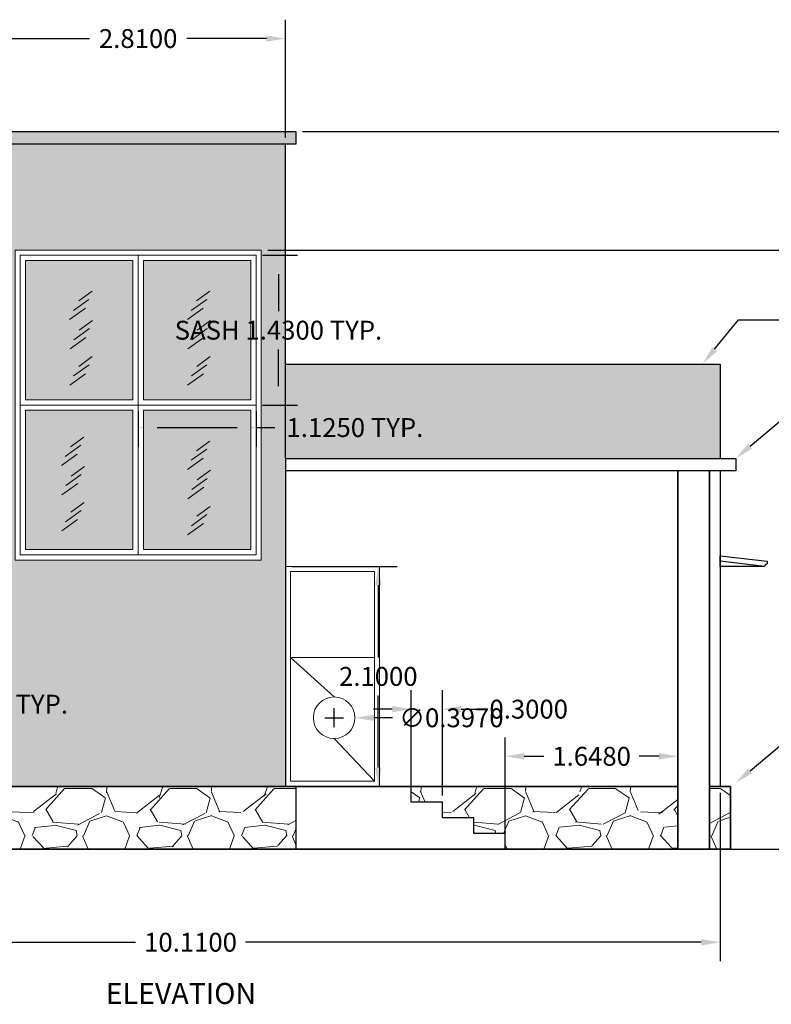
# Model space of a CAD drawing. Units: metres. Extents: x 5.2 to 41.7, y 12.2 to 37.4.
# Tile 2 of 6: x 12.3 to 19.4, y 28 to 37.4. Entities that reach past the tile are written whole.
import ezdxf
from ezdxf import colors
from ezdxf.entities.mleader import LeaderData, LeaderLine
from ezdxf.math import Vec2, Vec3

# ---------------------------------------------------------------- set-up
doc = ezdxf.new("R2010")
doc.units = ezdxf.units.M
doc.header["$MEASUREMENT"] = 0
for name, color, linetype, lineweight in [('A-ANNO-DIMS', 2, 'Continuous', 18), ('A-ANNO-TEXT', 3, 'Continuous', 18), ('A-COLS', 1, 'Continuous', 35), ('A-DOOR', 4, 'Continuous', 18), ('A-ELEV', 7, 'Continuous', 25), ('A-ELEV-PATT', 9, 'Continuous', 13), ('A-FLOR-PLIN', 7, 'Continuous', 25), ('A-FLOR-STRS', 7, 'Continuous', 25), ('A-GLAZ-PATT', 151, 'Continuous', 13), ('A-ROOF', 7, 'Continuous', 25), ('C-TOPO', 7, 'Continuous', 25)]:
    doc.layers.add(name, color=color, linetype=linetype, lineweight=lineweight)
doc.layers.add('A-GLAZ', color=51, linetype='Continuous', lineweight=18, true_color=0xf7f281)
doc.layers.add('A-PLIN-PATT', color=251, linetype='Continuous', lineweight=13, true_color=0x636466)
doc.styles.get("Standard").update_dxf_attribs({"font": 'arial.ttf'})
doc.dimstyles.get("Standard").update_dxf_attribs({"dimtxt": 0.18, "dimasz": 0.18, "dimexe": 0.18, "dimexo": 0.0625, "dimgap": 0.09, "dimtad": 0, "dimtih": 1, "dimtoh": 1, "dimdec": 4, "dimzin": 0, "dimdsep": 46, "dimtxsty": 'Standard', "dimcen": 0.09, "dimadec": 0, "dimazin": 0, "dimtfac": 1, "dimtdec": 4, "dimtofl": 0, "dimtmove": 0, "dimatfit": 3, "dimfxl": 1, "dimtolj": 1, "dimtzin": 0, "dimarcsym": 0})

# ---------------------------------------------------------------- blocks, each defined once
blk = doc.blocks.new('GLASS-REFLECTION')
for p, q in [((0.0369433649416564, 0.0871027572389061), (0.184953556568928, 0.1937230376420551)), ((0.08809580488861, 0.178305383476971), (0.2148507561325843, 0.2711338394228626)), ((0.000485723746344, -2.27863267348e-05), (0.1515279092010928, 0.1087816141597138))]:
    blk.add_line(p, q)
blk = doc.blocks.new('SASH-ELEV-TOWER')
for points in [[(-0.0004402787265363, 1.429717152800996), (1.12455972127346, 1.429717152800996), (1.12455972127346, -0.0002828471990028), (-0.0004402787265363, -0.0002828471990028)], [(0.0495597212734644, 1.379717152800999), (1.074559721273459, 1.379717152800999), (1.074559721273459, 0.0497171528009943), (0.0495597212734644, 0.0497171528009943)]]:
    blk.add_lwpolyline(points, close=True)
blk = doc.blocks.new('*D20')
at = {"layer": 'A-ANNO-DIMS', "color": 0, "lineweight": -2, "transparency": 16777216}
for p, q in [((14.58205972127346, 35.11471715280102), (14.91405972127346, 35.11471715280102)), ((14.73405972127346, 34.93471715280102), (14.73405972127346, 34.58284812142313)), ((14.73405972127346, 33.86471715280102), (14.73405972127346, 34.21658618417892)), ((14.58205972127346, 33.68471715280102), (14.91405972127346, 33.68471715280102))]:
    blk.add_line(p, q, dxfattribs=at)
at = {"layer": 'A-ANNO-DIMS', "color": 0, "lineweight": 25, "transparency": 16777216}
for points in [[(14.70405972127346, 34.93471715280102), (14.76405972127346, 34.93471715280102), (14.73405972127346, 35.11471715280102)], [(14.70405972127346, 33.86471715280102), (14.76405972127346, 33.86471715280102), (14.73405972127346, 33.68471715280102)]]:
    blk.add_solid(points, dxfattribs=at)
at = {"layer": 'Defpoints', "color": 0, "lineweight": 25, "transparency": 16777216}
for p in [(14.51955972127346, 35.11471715280102), (14.73405972127346, 35.11471715280102), (14.51955972127346, 33.68471715280102)]:
    blk.add_point(p, dxfattribs=at)
at = {"layer": 'A-ANNO-DIMS', "color": 0, "transparency": 16777216, "insert": (14.73405972127347, 34.39971715280102), "char_height": 0.18, "attachment_point": 5}
blk.add_mtext('\\A1;SASH 1.4300 TYP.', dxfattribs=at)
blk = doc.blocks.new('*D21')
at = {"layer": 'A-ANNO-DIMS', "color": 0, "lineweight": -2, "transparency": 16777216}
for p, q in [((13.39455972127345, 33.62221715280101), (13.39455972127345, 33.29021715280101)), ((14.51955972127345, 33.62221715280101), (14.51955972127345, 33.29021715280101)), ((13.57455972127345, 33.47021715280101), (14.33955972127345, 33.47021715280101)), ((14.51955972127345, 33.47021715280101), (14.69955972127345, 33.47021715280101))]:
    blk.add_line(p, q, dxfattribs=at)
at = {"layer": 'A-ANNO-DIMS', "color": 0, "lineweight": 25, "transparency": 16777216}
for points in [[(13.57455972127345, 33.50021715280101), (13.57455972127345, 33.44021715280101), (13.39455972127345, 33.47021715280101)], [(14.33955972127345, 33.50021715280101), (14.33955972127345, 33.44021715280101), (14.51955972127345, 33.47021715280101)]]:
    blk.add_solid(points, dxfattribs=at)
at = {"layer": 'Defpoints', "color": 0, "lineweight": 25, "transparency": 16777216}
for p in [(13.39455972127345, 33.68471715280101), (14.51955972127345, 33.68471715280101), (14.51955972127345, 33.47021715280101)]:
    blk.add_point(p, dxfattribs=at)
at = {"layer": 'A-ANNO-DIMS', "color": 0, "transparency": 16777216, "insert": (15.46388441431574, 33.47021715280101), "char_height": 0.18, "attachment_point": 5}
blk.add_mtext('\\A1;1.1250 TYP.', dxfattribs=at)
blk = doc.blocks.new('*D23')
at = {"layer": 'A-ANNO-DIMS', "color": 0, "lineweight": -2, "transparency": 16777216}
for p, q in [((10.56955972127346, 30.93221715280099), (10.56955972127346, 30.64971715280099)), ((11.11955972127346, 30.93221715280099), (11.11955972127346, 30.64971715280099)), ((10.74955972127346, 30.82971715280099), (10.93955972127346, 30.82971715280099)), ((11.11955972127346, 30.82971715280099), (11.29955972127346, 30.82971715280099))]:
    blk.add_line(p, q, dxfattribs=at)
at = {"layer": 'A-ANNO-DIMS', "color": 0, "lineweight": 25, "transparency": 16777216}
for points in [[(10.74955972127346, 30.85971715280099), (10.74955972127346, 30.79971715280099), (10.56955972127346, 30.82971715280099)], [(10.93955972127346, 30.85971715280099), (10.93955972127346, 30.79971715280099), (11.11955972127346, 30.82971715280099)]]:
    blk.add_solid(points, dxfattribs=at)
at = {"layer": 'Defpoints', "color": 0, "lineweight": 25, "transparency": 16777216}
for p in [(10.56955972127346, 30.99471715280099), (11.11955972127346, 30.99471715280099), (11.11955972127346, 30.82971715280099)]:
    blk.add_point(p, dxfattribs=at)
at = {"layer": 'A-ANNO-DIMS', "color": 0, "transparency": 16777216, "insert": (12.07235644705791, 30.82971715280099), "char_height": 0.18, "attachment_point": 5}
blk.add_mtext('\\A1;0.5500 TYP.', dxfattribs=at)
blk = doc.blocks.new('*D37')
at = {"layer": 'A-ANNO-DIMS', "color": 0, "lineweight": -2, "transparency": 16777216}
for p, q in [((8.83956, 29.982217), (8.83956, 28.377217)), ((18.94956, 29.982217), (18.94956, 28.377217)), ((9.01956, 28.557217), (13.36978510231924, 28.557217)), ((18.76956, 28.557217), (14.41933489768076, 28.557217))]:
    blk.add_line(p, q, dxfattribs=at)
at = {"layer": 'A-ANNO-DIMS', "color": 0, "lineweight": 25, "transparency": 16777216}
for points in [[(9.01956, 28.587217), (9.01956, 28.527217), (8.83956, 28.557217)], [(18.76956, 28.587217), (18.76956, 28.527217), (18.94956, 28.557217)]]:
    blk.add_solid(points, dxfattribs=at)
at = {"layer": 'Defpoints', "color": 0, "lineweight": 25, "transparency": 16777216}
for p in [(8.83956, 30.044717), (18.94956, 30.044717), (18.94956, 28.557217)]:
    blk.add_point(p, dxfattribs=at)
at = {"layer": 'A-ANNO-DIMS', "color": 0, "transparency": 16777216, "insert": (13.89456, 28.557217), "char_height": 0.18, "attachment_point": 5}
blk.add_mtext('\\A1;10.1100', dxfattribs=at)
blk = doc.blocks.new('*D38')
at = {"layer": 'A-ANNO-DIMS', "color": 0, "lineweight": -2, "transparency": 16777216}
for p, q in [((14.96206, 36.29607500000002), (22.42460000000001, 36.29607500000002)), ((22.24460000000001, 36.11607500000002), (22.24460000000001, 33.05229913778993)), ((22.24460000000001, 29.62471700000002), (22.24460000000001, 32.68849286221012)), ((21.4196, 29.44471700000002), (22.42460000000001, 29.44471700000002))]:
    blk.add_line(p, q, dxfattribs=at)
at = {"layer": 'A-ANNO-DIMS', "color": 0, "lineweight": 25, "transparency": 16777216}
for points in [[(22.21460000000001, 36.11607500000002), (22.27460000000001, 36.11607500000002), (22.24460000000001, 36.29607500000002)], [(22.21460000000001, 29.62471700000002), (22.27460000000001, 29.62471700000002), (22.24460000000001, 29.44471700000002)]]:
    blk.add_solid(points, dxfattribs=at)
at = {"layer": 'Defpoints', "color": 0, "lineweight": 25, "transparency": 16777216}
for p in [(14.89956, 36.29607500000002), (22.24460000000001, 36.29607500000002), (21.35710000000001, 29.44471700000002)]:
    blk.add_point(p, dxfattribs=at)
at = {"layer": 'A-ANNO-DIMS', "color": 0, "transparency": 16777216, "insert": (22.24460000000002, 32.87039600000001), "char_height": 0.18, "attachment_point": 5}
blk.add_mtext('\\A1;6.8514', dxfattribs=at)
blk = doc.blocks.new('*D41')
at = {"layer": 'A-ANNO-DIMS', "color": 0, "lineweight": -2, "transparency": 16777216}
for p, q in [((11.98956, 36.238575), (11.98956, 37.363575)), ((14.79956, 36.238575), (14.79956, 37.363575)), ((12.16956, 37.183575), (12.92970324693042, 37.183575)), ((14.61956, 37.183575), (13.85941675306957, 37.183575))]:
    blk.add_line(p, q, dxfattribs=at)
at = {"layer": 'A-ANNO-DIMS', "color": 0, "lineweight": 25, "transparency": 16777216}
for points in [[(12.16956, 37.213575), (12.16956, 37.153575), (11.98956, 37.183575)], [(14.61956, 37.213575), (14.61956, 37.153575), (14.79956, 37.183575)]]:
    blk.add_solid(points, dxfattribs=at)
at = {"layer": 'Defpoints', "color": 0, "lineweight": 25, "transparency": 16777216}
for p in [(14.79956, 37.183575), (11.98956, 36.176075), (14.79956, 36.176075)]:
    blk.add_point(p, dxfattribs=at)
at = {"layer": 'A-ANNO-DIMS', "color": 0, "transparency": 16777216, "insert": (13.39456, 37.183575), "char_height": 0.18, "attachment_point": 5}
blk.add_mtext('\\A1;2.8100', dxfattribs=at)
blk = doc.blocks.new('*D44')
at = {"layer": 'A-ANNO-DIMS', "color": 0, "lineweight": -2, "transparency": 16777216}
for p, q in [((14.86206000000001, 32.14471700000002), (15.86706000000001, 32.14471700000002)), ((15.68706000000001, 31.96471700000002), (15.68706000000001, 31.27662013778992)), ((15.68706000000001, 30.22471700000001), (15.68706000000001, 30.91281386221011)), ((14.86206000000001, 30.04471700000002), (15.86706000000001, 30.04471700000002))]:
    blk.add_line(p, q, dxfattribs=at)
at = {"layer": 'A-ANNO-DIMS', "color": 0, "lineweight": 25, "transparency": 16777216}
for points in [[(15.65706000000001, 31.96471700000002), (15.71706000000001, 31.96471700000002), (15.68706000000001, 32.14471700000002)], [(15.65706000000001, 30.22471700000001), (15.71706000000001, 30.22471700000001), (15.68706000000001, 30.04471700000002)]]:
    blk.add_solid(points, dxfattribs=at)
at = {"layer": 'Defpoints', "color": 0, "lineweight": 25, "transparency": 16777216}
for p in [(14.79956, 32.14471700000002), (14.79956, 30.04471700000002), (15.68706000000001, 30.04471700000002)]:
    blk.add_point(p, dxfattribs=at)
at = {"layer": 'A-ANNO-DIMS', "color": 0, "transparency": 16777216, "insert": (15.68706000000002, 31.094717), "char_height": 0.18, "attachment_point": 5}
blk.add_mtext('\\A1;2.1000', dxfattribs=at)
blk = doc.blocks.new('*D45')
at = {"layer": 'A-ANNO-DIMS', "color": 0, "lineweight": -2, "transparency": 16777216}
for p, q in [((14.96206, 36.29607500000002), (22.42460000000001, 36.29607500000002)), ((22.24460000000001, 36.11607500000002), (22.24460000000001, 35.91236052933155)), ((22.24460000000001, 35.34471700000003), (22.24460000000001, 35.54843147066851)), ((14.63206, 35.16471700000002), (22.42460000000001, 35.16471700000002))]:
    blk.add_line(p, q, dxfattribs=at)
at = {"layer": 'A-ANNO-DIMS', "color": 0, "lineweight": 25, "transparency": 16777216}
for points in [[(22.21460000000001, 36.11607500000002), (22.27460000000001, 36.11607500000002), (22.24460000000001, 36.29607500000002)], [(22.21460000000001, 35.34471700000003), (22.27460000000001, 35.34471700000003), (22.24460000000001, 35.16471700000002)]]:
    blk.add_solid(points, dxfattribs=at)
at = {"layer": 'Defpoints', "color": 0, "lineweight": 25, "transparency": 16777216}
for p in [(14.89956, 36.29607500000002), (22.24460000000001, 36.29607500000002), (14.56956, 35.16471700000002)]:
    blk.add_point(p, dxfattribs=at)
at = {"layer": 'A-ANNO-DIMS', "color": 0, "transparency": 16777216, "insert": (22.24460000000002, 35.73039600000001), "char_height": 0.18, "attachment_point": 5}
blk.add_mtext('\\A1;1.1314', dxfattribs=at)
blk = doc.blocks.new('*D76')
at = {"layer": 'A-ANNO-DIMS', "color": 0, "lineweight": -2, "transparency": 16777216}
for p, q in [((15.99956, 29.957217), (15.99956, 30.962217)), ((16.29956, 29.957217), (16.29956, 30.962217)), ((15.81956, 30.782217), (15.63956, 30.782217)), ((16.47956, 30.782217), (16.65956, 30.782217))]:
    blk.add_line(p, q, dxfattribs=at)
at = {"layer": 'A-ANNO-DIMS', "color": 0, "lineweight": 25, "transparency": 16777216}
for points in [[(15.81956, 30.812217), (15.81956, 30.752217), (15.99956, 30.782217)], [(16.47956, 30.812217), (16.47956, 30.752217), (16.29956, 30.782217)]]:
    blk.add_solid(points, dxfattribs=at)
at = {"layer": 'Defpoints', "color": 0, "lineweight": 25, "transparency": 16777216}
for p in [(16.29956, 30.782217), (15.99956, 29.894717), (16.29956, 29.894717)]:
    blk.add_point(p, dxfattribs=at)
at = {"layer": 'A-ANNO-DIMS', "color": 0, "transparency": 16777216, "insert": (17.12288196452933, 30.782217), "char_height": 0.18, "attachment_point": 5}
blk.add_mtext('\\A1;0.3000', dxfattribs=at)
blk = doc.blocks.new('*D77')
at = {"layer": 'A-ANNO-DIMS', "color": 0, "lineweight": -2, "transparency": 16777216}
for p, q in [((16.89956, 29.507217), (16.89956, 30.512217)), ((18.54752, 29.507217), (18.54752, 30.512217)), ((17.07956, 30.332217), (17.26869006821282, 30.332217)), ((18.36752, 30.332217), (18.17838993178717, 30.332217))]:
    blk.add_line(p, q, dxfattribs=at)
at = {"layer": 'A-ANNO-DIMS', "color": 0, "lineweight": 25, "transparency": 16777216}
for points in [[(17.07956, 30.362217), (17.07956, 30.302217), (16.89956, 30.332217)], [(18.36752, 30.362217), (18.36752, 30.302217), (18.54752, 30.332217)]]:
    blk.add_solid(points, dxfattribs=at)
at = {"layer": 'Defpoints', "color": 0, "lineweight": 25, "transparency": 16777216}
for p in [(18.54752, 30.332217), (16.89956, 29.444717), (18.54752, 29.444717)]:
    blk.add_point(p, dxfattribs=at)
at = {"layer": 'A-ANNO-DIMS', "color": 0, "transparency": 16777216, "insert": (17.72354, 30.332217), "char_height": 0.18, "attachment_point": 5}
blk.add_mtext('\\A1;1.6480', dxfattribs=at)
blk = doc.blocks.new('*D96')
at = {"layer": 'A-ANNO-DIMS', "color": 0, "lineweight": -2, "transparency": 16777216}
for p, q in [((15.26549799999999, 30.61012199999999), (15.26549799999999, 30.79012199999999)), ((15.175498, 30.700122), (15.355498, 30.700122)), ((15.82400293200936, 30.69977874616909), (15.64400296600468, 30.69988937308454))]:
    blk.add_line(p, q, dxfattribs=at)
at = {"layer": 'A-ANNO-DIMS', "color": 0, "lineweight": 25, "transparency": 16777216}
blk.add_solid([(15.64402140382392, 30.72988936741866), (15.64398452818543, 30.66988937875043), (15.464003, 30.7)], dxfattribs=at)
at = {"layer": 'Defpoints', "color": 0, "lineweight": 25, "transparency": 16777216}
for p in [(15.066993, 30.70024399999999), (15.464003, 30.7)]:
    blk.add_point(p, dxfattribs=at)
at = {"layer": 'A-ANNO-DIMS', "color": 0, "transparency": 16777216, "insert": (16.38524440540635, 30.69977874616909), "char_height": 0.18, "attachment_point": 5}
blk.add_mtext('\\A1;∅0.3970', dxfattribs=at)

msp = doc.modelspace()

# ---------------------------------------------------------------- hatches: boundary and pattern name
at = {"layer": 'A-ELEV-PATT'}
h = msp.add_hatch(color=256, dxfattribs=at)
h.dxf.hatch_style = 1
h.paths.add_polyline_path([(14.89955972127346, 36.29607479937437), (11.88955972127345, 36.29607479937437), (11.88955972127345, 36.17607479937438), (14.89955972127346, 36.17607479937438)])
h.paths.add_polyline_path([(11.98955972127346, 34.07607479937438), (8.839559721273464, 34.07607479937438), (8.839559721273464, 33.17607479937438), (11.98955972127346, 33.17607479937438)])
h.paths.add_polyline_path([(18.94955972127346, 34.07607479937438), (14.79955972127346, 34.07607479937438), (14.79955972127346, 33.17607479937438), (18.94955972127346, 33.17607479937438)])
h = msp.add_hatch(color=256, dxfattribs=at)
h.dxf.hatch_style = 1
h.paths.add_polyline_path([(14.79955972127346, 32.144717152801), (14.79955972127346, 33.17607479937438), (14.79955972127346, 36.17607479937438), (11.98955972127346, 36.17607479937438), (11.98955972127346, 33.17607479937438), (11.98955972127346, 30.04471715280099), (14.79955972127346, 30.044717152801)])
h.paths.add_polyline_path([(12.21955972127346, 32.204717152801), (12.21955972127346, 35.164717152801), (14.56955972127346, 35.164717152801), (14.56955972127346, 32.204717152801)], flags=16)
h.paths.add_polyline_path([(12.26955972127346, 32.254717152801), (12.26955972127346, 33.684717152801), (12.26955972127346, 35.114717152801), (13.39455972127346, 35.114717152801), (14.51955972127345, 35.114717152801), (14.51955972127345, 33.684717152801), (14.51955972127345, 32.254717152801), (13.39455972127346, 32.254717152801)], flags=0)
h.paths.add_polyline_path([(12.26955972127346, 32.25471715280099), (12.26955972127346, 35.114717152801), (14.51955972127346, 35.114717152801), (14.51955972127346, 32.25471715280099)], flags=0)
h.paths.add_polyline_path([(12.31955972127346, 32.304717152801), (12.31955972127346, 33.63471715280101), (13.34455972127346, 33.63471715280101), (13.34455972127346, 32.304717152801)], flags=0)
h.paths.add_polyline_path([(13.44455972127346, 32.304717152801), (13.44455972127346, 33.63471715280101), (14.46955972127345, 33.63471715280101), (14.46955972127345, 32.304717152801)], flags=0)
h.paths.add_polyline_path([(12.31955972127346, 33.734717152801), (12.31955972127346, 35.064717152801), (13.34455972127346, 35.064717152801), (13.34455972127346, 33.734717152801)], flags=0)
h.paths.add_polyline_path([(13.44455972127346, 33.734717152801), (13.44455972127346, 35.064717152801), (14.46955972127345, 35.064717152801), (14.46955972127345, 33.734717152801)], flags=0)
h = msp.add_hatch(color=256, dxfattribs=at)
h.dxf.hatch_style = 1
h.paths.add_polyline_path([(14.79955972127346, 32.144717152801), (14.79955972127346, 33.17607479937438), (14.79955972127346, 36.17607479937438), (11.98955972127346, 36.17607479937438), (11.98955972127346, 33.17607479937438), (11.98955972127346, 30.04471715280099), (14.79955972127346, 30.044717152801)])
h.paths.add_polyline_path([(12.21955972127346, 32.204717152801), (12.21955972127346, 35.164717152801), (14.56955972127346, 35.164717152801), (14.56955972127346, 32.204717152801)], flags=16)
h.paths.add_polyline_path([(13.39455972127346, 32.254717152801), (12.26955972127346, 32.254717152801), (12.26955972127346, 33.684717152801), (12.26955972127346, 35.114717152801), (13.39455972127346, 35.114717152801), (14.51955972127345, 35.114717152801), (14.51955972127345, 33.684717152801), (14.51955972127345, 32.254717152801)], flags=0)
h.paths.add_polyline_path([(12.26955972127346, 32.25471715280099), (12.26955972127346, 35.114717152801), (14.51955972127346, 35.114717152801), (14.51955972127346, 32.25471715280099)], flags=0)
h.paths.add_polyline_path([(13.44455972127346, 32.304717152801), (13.44455972127346, 33.63471715280101), (14.46955972127345, 33.63471715280101), (14.46955972127345, 32.304717152801)], flags=0)
h.paths.add_polyline_path([(13.34455972127346, 32.304717152801), (12.31955972127346, 32.304717152801), (12.31955972127346, 33.63471715280101), (13.34455972127346, 33.63471715280101)], flags=0)
h.paths.add_polyline_path([(13.44455972127346, 33.734717152801), (13.44455972127346, 35.064717152801), (14.46955972127345, 35.064717152801), (14.46955972127345, 33.734717152801)], flags=0)
h.paths.add_polyline_path([(13.34455972127346, 33.734717152801), (12.31955972127346, 33.734717152801), (12.31955972127346, 35.064717152801), (13.34455972127346, 35.064717152801)], flags=0)
at = {"layer": 'A-GLAZ-PATT'}
h = msp.add_hatch(color=256, dxfattribs=at)
h.dxf.hatch_style = 1
h.set_gradient(color1=(147, 149, 152), color2=(122, 175, 223))
h.paths.add_polyline_path([(13.34455972127346, 35.064717152801), (12.31955972127346, 35.064717152801), (12.31955972127346, 33.734717152801), (13.34455972127346, 33.734717152801)])
h.paths.add_polyline_path([(14.46955972127345, 33.63471715280101), (13.44455972127346, 33.63471715280101), (13.44455972127346, 32.304717152801), (14.46955972127345, 32.304717152801)])
h.paths.add_polyline_path([(14.46955972127345, 35.064717152801), (13.44455972127346, 35.064717152801), (13.44455972127346, 33.734717152801), (14.46955972127345, 33.734717152801)])
h.paths.add_polyline_path([(13.34455972127346, 33.63471715280101), (12.31955972127346, 33.63471715280101), (12.31955972127346, 32.304717152801), (13.34455972127346, 32.304717152801)])
at = {"layer": 'A-PLIN-PATT'}
h = msp.add_hatch(dxfattribs=at)
h.set_pattern_fill('GRAVEL', color=256)
h.set_pattern_definition([(228.012787504, (-11.19360896471565, -4.432464084464029), (-8.000000000000062, -9.000000000000004), [0.134536, -13.3190880470737]), (184.969740728, (-11.28360896471565, -4.532464084464029), (11.99999999999997, 1.000000000000035), [0.230868, -22.85592476122999]), (132.510447078, (-11.51360896471565, -4.55246408446403), (10.00000000000011, -10.99999999999986), [0.162788, -16.1160325960997]), (267.273689006, (-11.90360896471565, -4.80246408446403), (1.000000000000024, 20.00000000000002), [0.210238, -20.813558041629]), (292.833654178, (-11.91360896471565, -5.01246408446403), (-4.999999999999988, 12.00000000000003), [0.2061549999999999, -20.40937312808829]), (357.273689006, (-11.83360896471565, -5.202464084464029), (-20.00000000000002, 1.000000000000025), [0.210238, -20.813558041629]), (37.6942404667, (-11.62360896471565, -5.21246408446403), (-13, -9.999999999999973), [0.278029, -27.524848548916]), (72.2553283749, (-11.40360896471565, -5.04246408446403), (7.000000000000027, 22.00000000000001), [0.2624879999999999, -25.98632149681339]), (121.429565615, (-11.32360896471565, -4.79246408446403), (-8.00000000000002, 12.99999999999999), [0.21095, -20.884073109729]), (175.236358309, (-11.43360896471565, -4.612464084464029), (10.99999999999998, -1.000000000000037), [0.240832, -11.8007625787923]), (222.397437798, (-11.67360896471565, -4.59246408446403), (-11.99999999999996, -10.99999999999997), [0.311448, -30.8333750047949]), (138.814074834, (-10.91360896471565, -4.812464084464029), (-7.000000000000032, 6), [0.106301, -10.52384481273469]), (171.46923439, (-10.99360896471565, -4.74246408446403), (13, -1.999999999999995), [0.202237, -20.021511416157]), (225, (-11.19360896471565, -4.71246408446403), (-1e-16, -0.9999999999999328), [0.141421, -1.2727925623731]), (203.198590514, (-11.26360896471565, -4.59246408446403), (4.999999999999989, 1.999999999999975), [0.076158, -7.5396151058639]), (291.801409486, (-11.33360896471565, -4.622464084464029), (-0.9999999999996839, 3.000000000000102), [0.107703, -5.2774618071345]), (30.96375653209999, (-11.29360896471565, -4.722464084464029), (3.000000000000053, 1.999999999999979), [0.174929, -5.656022894845299]), (161.565051177, (-11.14360896471565, -4.63246408446403), (2.000000000000011, -0.9999999999999767), [0.1264909999999999, -3.035786660168398]), (16.389540334, (-11.91360896471565, -4.622464084464029), (9.999999999999966, 3.000000000000043), [0.1772, -17.5428451466694]), (70.3461759419, (-11.74360896471565, -4.572464084464029), (-4.00000000000122, -11.00000000000339), [0.148661, -14.717407747319]), (293.198590514, (-11.14360896471565, -4.432464084464029), (-1.99999999999997, 4.999999999999991), [0.152315, -7.4634581058639]), (343.610459666, (-11.08360896471565, -4.572464084464029), (-9.999999999999966, 3.000000000000043), [0.1771999999999999, -17.54284514666899]), (339.44395478, (-11.91360896471565, -5.242464084464029), (-5.000000000000036, 2.000000000000024), [0.1708799999999999, -8.373123745317496]), (294.775140569, (-11.75360896471565, -5.30246408446403), (-5.000000000000005, 11), [0.143178, -14.174643063276]), (66.8014094864, (-11.13360896471565, -5.432464084464029), (1.999999999999981, 4.999999999999969), [0.152315, -7.4634581058639]), (17.3540246363, (-11.07360896471565, -5.29246408446403), (-12.99999999999998, -3.999999999999962), [0.167631, -16.59542361424]), (69.4439547804, (-11.62360896471565, -5.432464084464029), (-2.000000000000007, -4.999999999999954), [0.08544, -8.458563745317496]), (101.3099324739999, (-11.19360896471565, -5.432464084464029), (-0.9999999999999637, 4.000000000000012), [0.05099, -5.048029513592799]), (165.963756532, (-11.20360896471565, -5.38246408446403), (2.999999999999958, -1.000000000000001), [0.206155, -3.9169506256177]), (186.009005957, (-11.40360896471565, -5.33246408446403), (10.00000000000004, 0.9999999999999831), [0.19105, -18.9139231745428]), (303.690067526, (-11.29360896471565, -4.812464084464029), (-0.9999999999999872, 1.999999999999985), [0.1442219999999999, -3.461329275463999]), (353.157226587, (-11.21360896471565, -4.932464084464029), (17.00000000000001, -2.000000000000052), [0.251794, -24.9275626240283]), (60.9453959009, (-10.96360896471565, -4.96246408446403), (-3.999999999999975, -6.999999999999976), [0.102956, -10.192674140987]), (90, (-10.91360896471565, -4.872464084464029), (-0.9999999999999998, 1), [0.06, -0.9399999999999998]), (120.256437164, (-11.42360896471565, -5.30246408446403), (4.000000000000008, -7.000000000000007), [0.138924, -13.7535199894498]), (48.01278750419999, (-11.49360896471565, -5.182464084464029), (8, 8.999999999999975), [0.269072, -13.1845520470737]), (0, (-11.31360896471565, -4.982464084464029), (1, 1), [0.26, -0.7400000000000001]), (325.304846469, (-11.05360896471565, -4.982464084464029), (10.00000000000014, -6.999999999999825), [0.1581139999999999, -15.65327430084199]), (254.0546040990001, (-10.92360896471565, -5.072464084464029), (-1.000000000000037, -4.000000000000004), [0.145602, -7.1345078892805]), (207.645975364, (-10.96360896471565, -5.21246408446403), (-18.99999999999995, -10.00000000000005), [0.237065, -23.4694741822594]), (175.42607874, (-11.17360896471565, -5.322464084464029), (-12.99999999999995, 1.000000000000001), [0.250799, -24.8290734079689])])
h.paths.add_polyline_path([(11.88955972127345, 30.04471715280099), (8.739559721273462, 30.04471715280099), (8.739559721273462, 29.44471715280099), (11.88955972127345, 29.44471715280099)])
h.paths.add_polyline_path([(14.89955972127346, 30.04471715280099), (11.88955972127345, 30.04471715280099), (11.88955972127345, 29.44471715280099), (14.89955972127346, 29.44471715280099)])
h.paths.add_polyline_path([(18.54752032864311, 30.04471715280099), (15.99955972127346, 30.04471715280099), (15.99955972127346, 29.89471715280099), (16.29955972127345, 29.89471715280099), (16.29955972127345, 29.74471715280099), (16.59955972127345, 29.74471715280099), (16.59955972127345, 29.59471715280099), (16.89955972127346, 29.59471715280099), (16.89955972127346, 29.44471715280099), (18.54752032864311, 29.44471715280099)])
h.paths.add_polyline_path([(19.04955972127346, 30.04471715280099), (18.84752032864312, 30.04471715280099), (18.84752032864312, 29.44471715280099), (19.04955972127346, 29.44471715280099)])

# ---------------------------------------------------------------- linework, layer by layer
at = {"layer": 'A-COLS'}
for p, q in [((18.54752032864311, 33.05607479937438), (18.54752032864311, 29.44471715280099)), ((18.84752032864312, 33.05607479937438), (18.84752032864312, 29.44471715280099))]:
    msp.add_line(p, q, dxfattribs=at)
at = {"layer": 'A-DOOR'}
for p, q in [((15.265498299819, 30.89862662219574), (14.84955972127346, 31.27385218716647)), ((15.265498299819, 30.50161798436073), (15.64955972127347, 30.09471715280099))]:
    msp.add_line(p, q, dxfattribs=at)
for points in [[(14.79955972127346, 32.144717152801), (15.69955972127347, 32.144717152801), (15.69955972127347, 30.04471715280099), (14.79955972127346, 30.04471715280099)], [(14.84955972127346, 32.094717152801), (15.64955972127347, 32.094717152801), (15.64955972127347, 30.09471715280099), (14.84955972127346, 30.09471715280099)], [(14.84955972127346, 32.094717152801), (15.64955972127347, 32.094717152801), (15.64955972127347, 31.27385218716647), (14.84955972127346, 31.27385218716647)]]:
    msp.add_lwpolyline(points, close=True, dxfattribs=at)
msp.add_circle((15.265498299819, 30.70012230327824), 0.1985043189175042, dxfattribs=at)
at = {"layer": 'A-ELEV'}
for p, q in [((14.79955972127346, 33.17607479937438), (14.79955972127346, 36.17607479937438)), ((14.79955972127346, 34.07607479937438), (18.94955972127346, 34.07607479937438)), ((18.94955972127346, 34.07607479937438), (18.94955972127346, 33.17607479937438)), ((14.79955972127346, 33.17607479937438), (14.79955972127346, 30.04471715280099)), ((18.94955972127346, 33.05607479937438), (18.94955972127346, 30.04471715280099))]:
    msp.add_line(p, q, dxfattribs=at)
at = {"layer": 'A-FLOR-PLIN'}
for p, q in [((18.54752032864311, 30.044717152801), (8.739559721273462, 30.04471715280099)), ((14.89955972127346, 30.04471715280099), (14.89955972127346, 29.44471715280099)), ((19.04955972127346, 30.04471715280099), (18.84752032864312, 30.044717152801)), ((19.04955972127346, 29.44471715280099), (19.04955972127346, 30.04471715280099)), ((8.739559721273462, 29.44471715280099), (19.04955972127346, 29.44471715280099))]:
    msp.add_line(p, q, dxfattribs=at)
msp.add_lwpolyline([(18.84752032864312, 30.04471715280099), (19.04955972127346, 30.04471715280099), (19.04955972127346, 29.44471715280099), (8.739559721273462, 29.44471715280099), (8.739559721273462, 30.04471715280099), (18.54752032864311, 30.04471715280099)], dxfattribs=at)
at = {"layer": 'A-FLOR-STRS'}
for p, q in [((15.99955972127346, 29.89471715280099), (15.99955972127346, 30.04471715280099)), ((16.29955972127345, 29.89471715280099), (15.99955972127346, 29.89471715280099)), ((16.29955972127345, 29.74471715280099), (16.29955972127345, 29.89471715280099)), ((16.59955972127345, 29.74471715280099), (16.29955972127345, 29.74471715280099)), ((16.59955972127345, 29.59471715280099), (16.59955972127345, 29.74471715280099)), ((16.89955972127346, 29.59471715280099), (16.59955972127345, 29.59471715280099)), ((16.89955972127346, 29.44471715280099), (16.89955972127346, 29.59471715280099))]:
    msp.add_line(p, q, dxfattribs=at)
at = {"layer": 'A-GLAZ'}
for points in [[(12.21955972127346, 35.164717152801), (14.56955972127346, 35.164717152801), (14.56955972127346, 32.204717152801), (12.21955972127346, 32.204717152801)], [(12.26955972127346, 35.114717152801), (14.51955972127346, 35.114717152801), (14.51955972127346, 32.25471715280099), (12.26955972127346, 32.25471715280099)]]:
    msp.add_lwpolyline(points, close=True, dxfattribs=at)
at = {"layer": 'A-ROOF'}
for p, q in [((14.79955972127346, 33.17607479937438), (18.94955972127346, 33.17607479937438)), ((18.94955972127346, 33.17607479937438), (19.09955972127345, 33.17607479937438)), ((19.09955972127345, 33.17607479937438), (19.09955972127345, 33.05607479937438)), ((18.94955972127346, 33.05607479937438), (14.79955972127346, 33.05607479937438)), ((19.09955972127345, 33.05607479937438), (18.94955972127346, 33.05607479937438)), ((18.94955972127346, 32.24471715280099), (19.39955972127345, 32.19471715280099)), ((19.37455972127345, 32.144717152801), (18.94955972127346, 32.19471715280099))]:
    msp.add_line(p, q, dxfattribs=at)
msp.add_lwpolyline([(11.88955972127345, 36.29607479937437), (14.89955972127346, 36.29607479937437), (14.89955972127346, 36.17607479937438), (11.88955972127345, 36.17607479937438)], close=True, dxfattribs=at)
for points in [[(19.37455972127345, 32.144717152801), (18.94955972127346, 32.144717152801), (18.94955972127346, 32.24471715280099)], [(19.39955972127345, 32.19471715280099), (19.39955972127345, 32.16971715280099)]]:
    msp.add_lwpolyline(points, dxfattribs=at)
msp.add_arc((19.39955972127345, 32.144717152801), 0.0249999999999986, 90, 180, dxfattribs=at)
at = {"layer": 'C-TOPO'}
msp.add_line((19.04955972127346, 29.44471715280099), (21.35710035431744, 29.44471715280099), dxfattribs=at)

# ---------------------------------------------------------------- block references
at = {"layer": 'A-GLAZ'}
for p in [(12.27, 33.685), (13.39499999999999, 33.68500000000001), (12.27, 32.255), (13.39499999999999, 32.25500000000001)]:
    msp.add_blockref('SASH-ELEV-TOWER', p, dxfattribs=at)
at = {"layer": 'A-GLAZ-PATT'}
for p in [(12.73902390578852, 34.50035240824278), (13.86402390578853, 34.50035240824278), (12.74396391638485, 34.22141176932402), (13.86896391638485, 34.22141176932402), (12.74149391108669, 33.87582149357374), (13.86649391108669, 33.87582149357374), (12.66177894354373, 33.10785418506127), (13.86402390578852, 33.07035240824278), (12.66671895414006, 32.8289135461425), (13.86896391638485, 32.79141176932402), (12.6642489488419, 32.48332327039222), (13.86649391108669, 32.44582149357374)]:
    msp.add_blockref('GLASS-REFLECTION', p, dxfattribs=at)

# ---------------------------------------------------------------- texts
at = {"layer": 'A-ANNO-TEXT', "insert": (12.39140313616877, 28.16833005504314), "char_height": 0.2, "attachment_point": 1}
msp.add_mtext_dynamic_manual_height_columns('\\pxqc;{ELEVATION }', width=2.822089916971947, gutter_width=1, heights=[0], dxfattribs=at)

# ---------------------------------------------------------------- dimensions: what is measured, and where the dimension line sits
at = {"layer": 'A-ANNO-DIMS'}
for base, p1, p2, picture, middle in [((14.79956, 37.183575), (11.98956, 36.176075), (14.79956, 36.176075), '*D41', (13.39456, 37.183575)), ((16.29956, 30.782217), (15.99956, 29.894717), (16.29956, 29.894717), '*D76', (17.12288196452933, 30.782217)), ((18.54752, 30.332217), (16.89956, 29.444717), (18.54752, 29.444717), '*D77', (17.72354, 30.332217)), ((18.94956, 28.557217), (8.83956, 30.044717), (18.94956, 30.044717), '*D37', (13.89456, 28.557217))]:
    dim = msp.add_linear_dim(base=base, p1=p1, p2=p2, dimstyle='Standard', override={"dimdec": 4, "dimlfac": 1, "dimrnd": 0, "dimzin": 0, "dimdsep": 46, "dimlunit": 2}, dxfattribs=at)
    dim.commit()
    dim.dimension.update_dxf_attribs({"geometry": picture, "text_midpoint": middle})
for base, p1, p2, angle, picture, middle in [((22.24460000000001, 36.29607500000002), (14.56956, 35.164717), (14.89956, 36.296075), 90, '*D45', (22.24460000000002, 35.73039600000001)), ((22.24460000000001, 36.29607500000002), (21.3571, 29.444717), (14.89956, 36.296075), 90, '*D38', (22.24460000000002, 32.87039600000001)), ((15.68706000000001, 30.04471700000002), (14.79956, 32.144717), (14.79956, 30.044717), 270, '*D44', (15.68706000000002, 31.094717))]:
    dim = msp.add_linear_dim(base=base, p1=p1, p2=p2, angle=angle, dimstyle='Standard', override={"dimdec": 4, "dimlfac": 1, "dimrnd": 0, "dimzin": 0, "dimdsep": 46, "dimlunit": 2}, dxfattribs=at)
    dim.commit()
    dim.dimension.update_dxf_attribs({"geometry": picture, "text_midpoint": middle})
dim = msp.add_linear_dim(base=(14.73405972127346, 35.11471715280102), p1=(14.51955972127345, 33.68471715280101), p2=(14.51955972127345, 35.11471715280101), angle=90, text='SASH <> TYP.', dimstyle='Standard', override={"dimdec": 4, "dimlfac": 1, "dimrnd": 0, "dimzin": 0, "dimdsep": 46, "dimlunit": 2}, dxfattribs=at)
dim.commit()
dim.dimension.update_dxf_attribs({"geometry": '*D20', "text_midpoint": (14.73405972127347, 34.39971715280102)})
for base, p1, p2, picture, middle in [((14.51955972127345, 33.47021715280101), (13.39455972127345, 33.68471715280101), (14.51955972127345, 33.68471715280101), '*D21', (15.46388441431574, 33.47021715280101)), ((11.11955972127346, 30.82971715280099), (10.56955972127346, 30.99471715280099), (11.11955972127346, 30.99471715280099), '*D23', (12.07235644705791, 30.82971715280099))]:
    dim = msp.add_linear_dim(base=base, p1=p1, p2=p2, text='<> TYP.', dimstyle='Standard', override={"dimdec": 4, "dimlfac": 1, "dimrnd": 0, "dimzin": 0, "dimdsep": 46, "dimlunit": 2}, dxfattribs=at)
    dim.commit()
    dim.dimension.update_dxf_attribs({"geometry": picture, "text_midpoint": middle})
dim = msp.add_diameter_dim_2p(p1=(15.066993, 30.70024399999999), p2=(15.464003, 30.7), dimstyle='Standard', override={"dimdec": 4, "dimlfac": 1, "dimrnd": 0, "dimzin": 0, "dimdsep": 46, "dimlunit": 2}, dxfattribs=at)
dim.commit()
dim.dimension.update_dxf_attribs({"geometry": '*D96', "text_midpoint": (15.82400293200936, 30.69977874616909)})

# ---------------------------------------------------------------- leaders
at = {"layer": 'A-ANNO-TEXT'}
ml = msp.add_multileader_mtext('Standard', dxfattribs=at)
ml.set_content('Parapet Wall  0.9 m  ', color=256)
ml.set_leader_properties()
ml.build(insert=Vec2(0, 0))
ml.multileader.update_dxf_attribs({"dogleg_length": 0.36, "arrow_head_size": 0.18})
ctx = ml.context
ctx.base_point, ctx.char_height, ctx.arrow_head_size, ctx.landing_gap_size, ctx.plane_origin = Vec3(20.00371874595419, 34.49999431774039), 0.18, 0.18, 0.09, Vec3(18.71194832135768, 33.97238036568555)
notes = []
notes.append((ctx, [(0, (1, 1, 0), (19.12674881396788, 34.49999431774039), (1, 0), 0.8769699319863098, [(0, [(18.78337575428395, 34.07757905478835)], 0, [])])]))
ctx.mtext.insert, ctx.mtext.flow_direction = Vec3(20.09371874595419, 34.61498067517559), 5
ml = msp.add_multileader_mtext('Standard', dxfattribs=at)
ml.set_content('Slab 0.12 m   ', color=256)
ml.set_leader_properties()
ml.build(insert=Vec2(0, 0))
ml.multileader.update_dxf_attribs({"dogleg_length": 0.36, "arrow_head_size": 0.18})
ctx = ml.context
ctx.base_point, ctx.char_height, ctx.arrow_head_size, ctx.landing_gap_size, ctx.plane_origin = Vec3(20.41301654737379, 33.54317992515984), 0.18, 0.18, 0.09, Vec3(18.94270675488576, 32.33032346424838)
notes.append((ctx, [(0, (1, 1, 0), (19.53604661538747, 33.54317992515984), (1, 0), 0.8769699319863098, [(0, [(19.09955972127345, 33.17607479937438)], 0, [])])]))
ctx.mtext.insert, ctx.mtext.flow_direction = Vec3(20.50301654737379, 33.63471471370008), 5
ml = msp.add_multileader_mtext('Standard', dxfattribs=at)
ml.set_content('Plinth 0.6 m   ', color=256)
ml.set_leader_properties()
ml.build(insert=Vec2(0, 0))
ml.multileader.update_dxf_attribs({"dogleg_length": 0.36, "arrow_head_size": 0.18})
ctx = ml.context
ctx.base_point, ctx.char_height, ctx.arrow_head_size, ctx.landing_gap_size, ctx.plane_origin = Vec3(20.41301654737379, 30.44541204035794), 0.18, 0.18, 0.09, Vec3(18.94270675488576, 29.23255557944648)
notes.append((ctx, [(0, (1, 1, 0), (19.53604661538747, 30.44541204035794), (1, 0), 0.8769699319863098, [(0, [(19.09955972127345, 30.07830691457248)], 0, [])])]))
ctx.mtext.insert, ctx.mtext.flow_direction = Vec3(20.50301654737379, 30.53694682889818), 5
for ctx, leaders in notes:
    for number, flags, end, landing, length, lines in leaders:
        leader = LeaderData()
        leader.index, (leader.has_last_leader_line, leader.has_dogleg_vector, leader.attachment_direction) = number, flags
        leader.last_leader_point, leader.dogleg_vector, leader.dogleg_length = Vec3(end), Vec3(landing), length
        for number, points, colour, breaks in lines:
            line = LeaderLine()
            line.index, line.vertices, line.color, line.breaks = number, Vec3.list(points), colors.encode_raw_color(colour), breaks
            leader.lines.append(line)
        ctx.leaders.append(leader)

doc.saveas('drawing.dxf')
